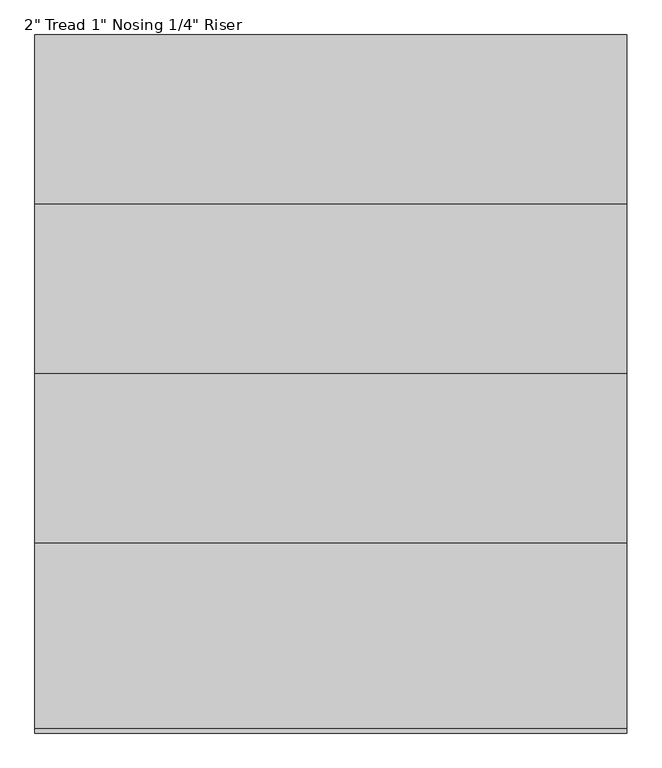
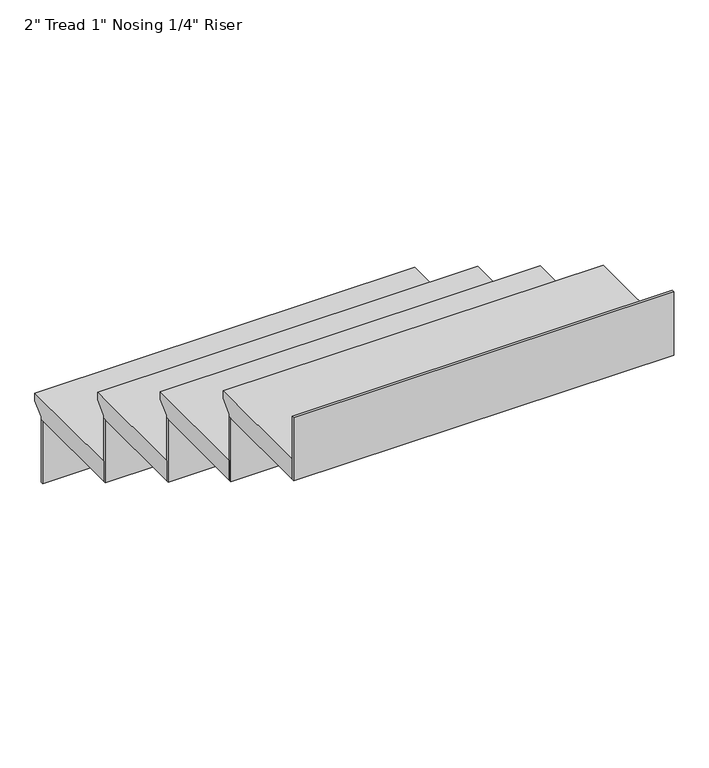
"""IFC4 building model written with IfcOpenShell, lengths in millimetres: stair flight geometry."""

from ifc_helpers import new_model, si_unit, frame, origin, place, context, project, spatial, polyline, outline, extrude, source, transform, mapped, element, save


def stair_flight_157d76c2(model_context):
    return source(origin(), model_context, "Body", "SweptSolid", [
        extrude(outline(polyline([(10449.3013837, 2406.3157895), (10736.3412275, 2406.3157895), (10736.3412275, 2387.2657895), (10710.9412275, 2361.8657895), (10710.9412275, 2355.5157895), (10449.3013837, 2355.5157895), (10449.3013837, 2406.3157895)])), frame((-11648.3149392, 0.0, 0.0), z_axis=(1.0, 0.0, 0.0), x_axis=(0.0, 1.0, 0.0)), (0.0, 0.0, 1.0), 914.4),
        extrude(outline(polyline([(-11648.3149392, 10704.5912275), (-11648.3149392, 10710.9412275), (-10733.9149392, 10710.9412275), (-10733.9149392, 10704.5912275), (-11648.3149392, 10704.5912275)])), frame((0.0, 0.0, 2195.0947368), z_axis=(0.0, 0.0, 1.0), x_axis=(1.0, 0.0, 0.0)), (0.0, 0.0, 1.0), 160.4210526),
        extrude(outline(polyline([(-11648.3149392, 10442.9513837), (-11648.3149392, 10449.3013837), (-10733.9149392, 10449.3013837), (-10733.9149392, 10442.9513837), (-11648.3149392, 10442.9513837)])), frame((0.0, 0.0, 2355.5157895), z_axis=(0.0, 0.0, 1.0), x_axis=(1.0, 0.0, 0.0)), (0.0, 0.0, 1.0), 160.4210526),
        extrude(outline(polyline([(10187.66154, 2566.7368421), (10474.7013837, 2566.7368421), (10474.7013837, 2547.6868421), (10449.3013837, 2522.2868421), (10449.3013837, 2515.9368421), (10187.66154, 2515.9368421), (10187.66154, 2566.7368421)])), frame((-11648.3149392, 0.0, 0.0), z_axis=(1.0, 0.0, 0.0), x_axis=(0.0, 1.0, 0.0)), (0.0, 0.0, 1.0), 914.4),
        extrude(outline(polyline([(-11648.3149392, 10181.31154), (-11648.3149392, 10187.66154), (-10733.9149392, 10187.66154), (-10733.9149392, 10181.31154), (-11648.3149392, 10181.31154)])), frame((0.0, 0.0, 2515.9368421), z_axis=(0.0, 0.0, 1.0), x_axis=(1.0, 0.0, 0.0)), (0.0, 0.0, 1.0), 160.4210526),
        extrude(outline(polyline([(9926.0216962, 2727.1578947), (10213.06154, 2727.1578947), (10213.06154, 2708.1078947), (10187.66154, 2682.7078947), (10187.66154, 2676.3578947), (9926.0216962, 2676.3578947), (9926.0216962, 2727.1578947)])), frame((-11648.3149392, 0.0, 0.0), z_axis=(1.0, 0.0, 0.0), x_axis=(0.0, 1.0, 0.0)), (0.0, 0.0, 1.0), 914.4),
        extrude(outline(polyline([(-11648.3149392, 9919.6716962), (-11648.3149392, 9926.0216962), (-10733.9149392, 9926.0216962), (-10733.9149392, 9919.6716962), (-11648.3149392, 9919.6716962)])), frame((0.0, 0.0, 2676.3578947), z_axis=(0.0, 0.0, 1.0), x_axis=(1.0, 0.0, 0.0)), (0.0, 0.0, 1.0), 160.4210526),
        extrude(outline(polyline([(-11648.3149392, 9658.0318525), (-11648.3149392, 9664.3818525), (-10733.9149392, 9664.3818525), (-10733.9149392, 9658.0318525), (-11648.3149392, 9658.0318525)])), frame((0.0, 0.0, 2836.7789474), z_axis=(0.0, 0.0, 1.0), x_axis=(1.0, 0.0, 0.0)), (0.0, 0.0, 1.0), 160.4210526),
        extrude(outline(polyline([(9664.3818525, 2887.5789474), (9951.4216962, 2887.5789474), (9951.4216962, 2868.5289474), (9926.0216962, 2843.1289474), (9926.0216962, 2836.7789474), (9664.3818525, 2836.7789474), (9664.3818525, 2887.5789474)])), frame((-11648.3149392, 0.0, 0.0), z_axis=(1.0, 0.0, 0.0), x_axis=(0.0, 1.0, 0.0)), (0.0, 0.0, 1.0), 914.4),
    ])


if __name__ == "__main__":
    model = new_model("IFC4")
    model_context = context("Model", 3, world=origin())
    ifc_project = project(units=[si_unit("LENGTHUNIT", "METRE", prefix="MILLI")], contexts=[model_context])
    site = spatial("IfcSite", under=ifc_project)
    building = spatial("IfcBuilding", under=site)
    placement = place(None, origin())
    stair_flight_shape = stair_flight_157d76c2(model_context)
    element("IfcStairFlight", 1, ObjectType="2\" Tread 1\" Nosing 1/4\" Riser", at=placement, inside=building, context=model_context, shape_type="MappedRepresentation", body=[
        mapped(stair_flight_shape, transform((0.0, 0.0, 0.0), x_axis=(1.0, 0.0, 0.0), y_axis=(0.0, 1.0, 0.0), z_axis=(0.0, 0.0, 1.0))),
    ])
    save(model, "model.ifc")
